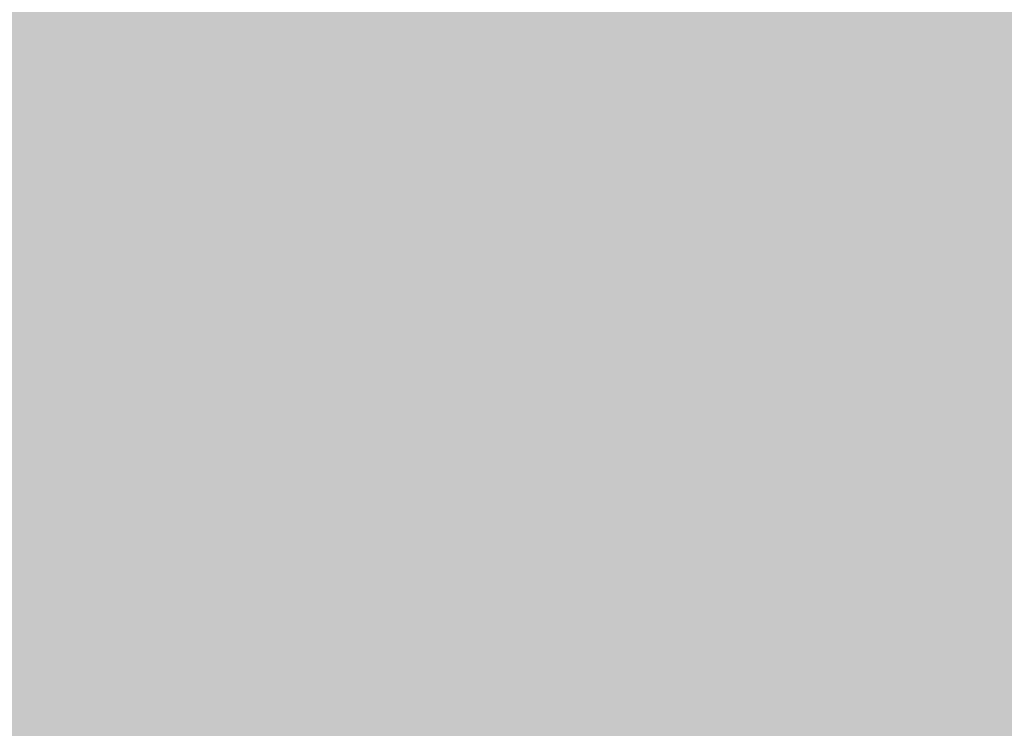
# Model space of a CAD drawing. Units: feet. Extents: x 3168 to 4724, y 827 to 1477.
# Tile 123 of 256: x 3298.685 to 3300.858, y 1096.781 to 1098.344. Entities that reach past the tile are written whole.
import ezdxf

# ---------------------------------------------------------------- set-up
doc = ezdxf.new("R2010")
doc.units = ezdxf.units.FT
doc.layers.add('A-ELEV-PATT', color=8, linetype='Continuous', lineweight=13)

msp = doc.modelspace()

# ---------------------------------------------------------------- hatches: boundary and pattern name
at = {"layer": 'A-ELEV-PATT'}
h = msp.add_hatch(color=256, dxfattribs=at)
h.dxf.hatch_style = 1
edge = h.paths.add_edge_path()
edge.add_ellipse((3552.9058, 979.2201), major_axis=(36.7449, 0), ratio=0.4848485, start_angle=0, end_angle=360)
edge = h.paths.add_edge_path()
edge.add_ellipse((3559.8916, 929.2523), major_axis=(36.7449, 0), ratio=0.4848485, start_angle=0, end_angle=360)
edge = h.paths.add_edge_path()
edge.add_line((3299.3168, 1198.6061), (3479.9167, 1198.6061))
edge.add_line((3479.9167, 1198.6061), (3479.9167, 1209.8686))
edge.add_spline(control_points=[(3479.9167, 1209.8686), (3464.3012, 1209.8686), (3448.6856, 1209.8686), (3410.9491, 1209.8686), (3388.8282, 1209.8686), (3355.6469, 1209.8686), (3344.5864, 1209.8686), (3327.9957, 1209.8686), (3322.4655, 1209.8686), (3314.1702, 1209.8686), (3311.4051, 1209.8686), (3307.2574, 1209.8686), (3305.8748, 1209.8686), (3303.801, 1209.8686), (3303.1097, 1209.8686), (3302.0728, 1209.8686), (3301.7272, 1209.8686), (3301.2087, 1209.8686), (3301.0359, 1209.8686), (3300.7767, 1209.8686), (3300.6903, 1209.8686), (3300.5606, 1209.8686), (3300.5174, 1209.8686), (3300.4526, 1209.8686), (3300.431, 1209.8686), (3300.3986, 1209.8686), (3300.3878, 1209.8686), (3300.3662, 1209.8686), (3300.3457, 1209.8686), (3300.3455, 1209.8686), (3300.3455, 1209.8686), (3300.3433, 1209.8686), (3300.3411, 1209.8686), (3300.3379, 1209.8686), (3300.3368, 1209.8686), (3300.3339, 1209.8686), (3300.3321, 1209.8686), (3300.3255, 1209.8686), (3300.3207, 1209.8686), (3300.3109, 1209.8686), (3300.306, 1209.8686), (3300.2905, 1209.8686), (3300.28, 1209.8686), (3300.2324, 1209.8688), (3300.1953, 1209.869), (3299.9511, 1209.8706), (3299.7448, 1209.8743), (3299.4368, 1209.8833), (3299.3344, 1209.8868), (3299.1811, 1209.8929), (3299.13, 1209.8951), (3298.6522, 1209.9168), (3298.2295, 1209.9457), (3297.6016, 1210.0024), (3297.3934, 1210.0235), (3297.0827, 1210.0583), (3296.9793, 1210.0705), (3296.293, 1210.1549), (3295.7181, 1210.2434), (3294.8687, 1210.3989), (3294.5877, 1210.4545), (3294.1693, 1210.5433), (3294.0304, 1210.5739), (3291.7071, 1211.1012), (3289.6536, 1211.8134), (3285.7763, 1213.564), (3283.9514, 1214.6035), (3280.5122, 1216.9801), (3278.8972, 1218.3176), (3276.3799, 1220.8295), (3275.416, 1221.9177), (3274.0393, 1223.7077), (3273.581, 1224.3495), (3273.1432, 1225.0163)], knot_values=[39.119033, 39.119033, 39.119033, 39.119033, 39.286353, 39.286353, 39.523379, 39.523379, 39.641892, 39.641892, 39.701148, 39.701148, 39.730777, 39.730777, 39.745591, 39.745591, 39.752998, 39.752998, 39.756701, 39.756701, 39.758553, 39.758553, 39.759479, 39.759479, 39.759942, 39.759942, 39.760173, 39.760173, 39.760289, 39.760289, 39.760405, 39.760405, 39.760463, 39.760463, 39.763389, 39.763389, 39.764851, 39.764851, 39.767304, 39.767304, 39.773825, 39.773825, 39.78057, 39.78057, 39.79477, 39.79477, 39.845194, 39.845194, 40.126715, 40.126715, 40.267476, 40.267476, 40.337856, 40.337856, 40.927023, 40.927023, 41.221606, 41.221606, 41.368898, 41.368898, 42.202622, 42.202622, 42.619485, 42.619485, 42.827916, 42.827916, 46.118323, 46.118323, 49.408731, 49.408731, 52.699139, 52.699139, 54.927489, 54.927489, 56.104228, 56.104228, 56.104228, 56.104228], weights=[1, 1, 1, 1, 1, 1, 1, 1, 1, 1, 1, 1, 1, 1, 1, 1, 1, 1, 1, 1, 1, 1, 1, 1, 1, 1, 1, 1, 1, 1, 1, 1, 1, 1, 1, 1, 1, 1, 1, 1, 1, 1, 1, 1, 1, 1, 1, 1, 1, 1, 1, 1, 1, 1, 1, 1, 1, 1, 1, 1, 1, 1, 1, 1, 1, 1, 1, 1, 1, 1, 1, 1, 1, 1], degree=3, periodic=0)
edge.add_line((3273.1432, 1225.0163), (3273.1432, 1099.0163))
edge.add_line((3273.1432, 1099.0163), (3299.3168, 1099.0163))
edge.add_line((3299.3168, 1099.0163), (3299.3168, 1198.6061))
edge = h.paths.add_edge_path()
edge.add_line((3304.7584, 1324.1581), (3479.9167, 1324.1581))
edge.add_line((3479.9167, 1324.1581), (3479.9167, 1335.7146))
edge.add_line((3479.9167, 1335.7146), (3269.1616, 1335.7146))
edge.add_spline(control_points=[(3269.1616, 1335.7146), (3264.0242, 1335.7146), (3258.3641, 1328.9582), (3259.2643, 1323.9003)], knot_values=[0, 0, 0, 0, 15.412191, 15.412191, 15.412191, 15.412191], degree=3, periodic=0)
edge.add_line((3259.2643, 1323.9003), (3265.5168, 1288.7691))
edge.add_line((3265.5168, 1288.7691), (3275.2651, 1261.5456))
edge.add_line((3275.2651, 1261.5456), (3304.7584, 1261.5456))
edge.add_line((3304.7584, 1261.5456), (3304.7584, 1324.1581))
h = msp.add_hatch(color=256, dxfattribs=at)
h.dxf.hatch_style = 1
h.paths.add_polyline_path([(3384.5252, 1099.0163), (3335.0292, 1099.0163), (3299.3168, 1099.0163), (3273.1432, 1099.0163), (3217.5654, 1099.0163), (3168.0693, 827.1163), (3335.0292, 827.1163)])

doc.saveas('drawing.dxf')
